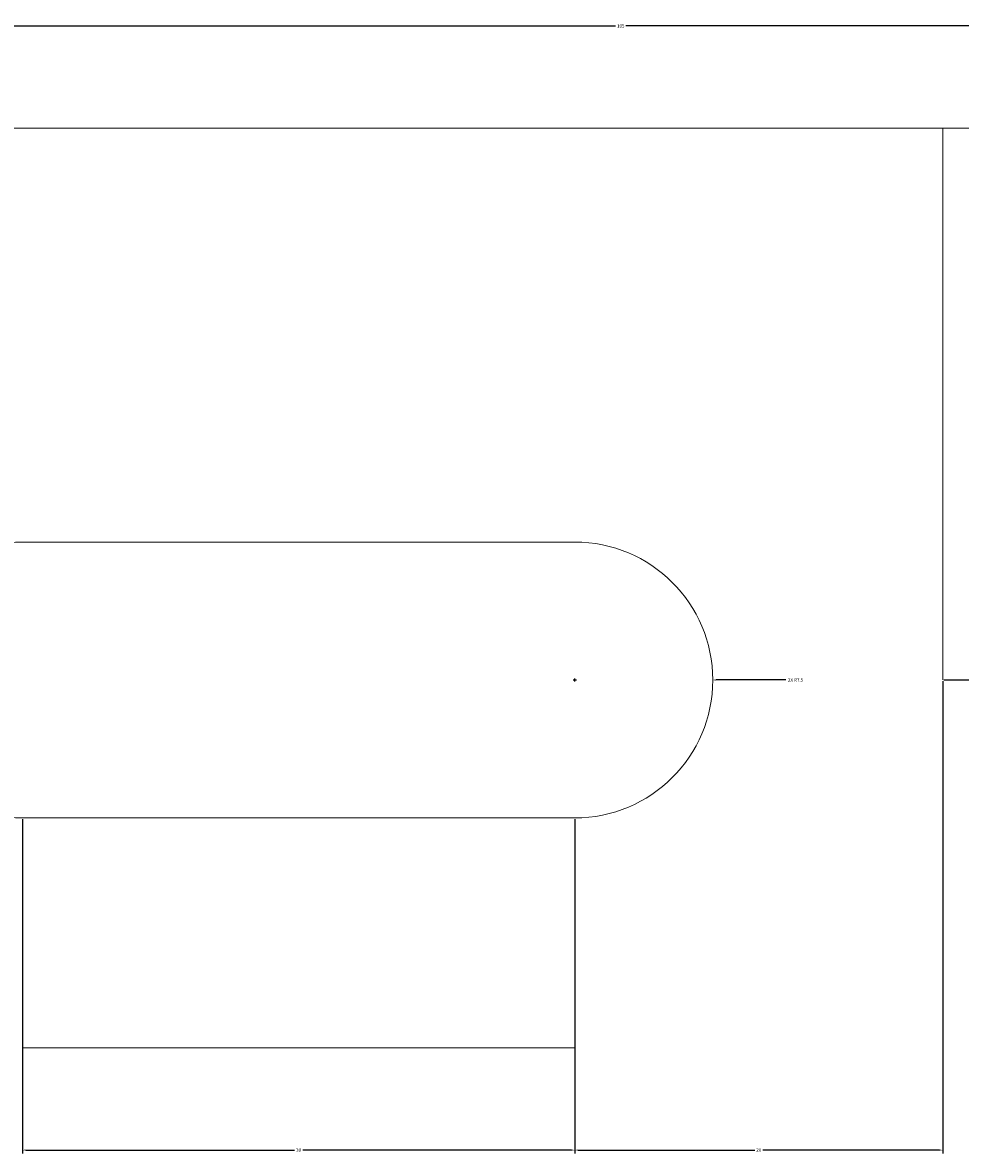
# Model space of a CAD drawing. Units: millimetres. Extents: x 88 to 204, y -56 to 6.
# Tile 2 of 3: x 114 to 165, y -56 to 6. Entities that reach past the tile are written whole.
import ezdxf

# ---------------------------------------------------------------- set-up
doc = ezdxf.new("R2010")
doc.units = ezdxf.units.MM
doc.layers.add('M-CONS', color=8, linetype='Continuous', lineweight=13)
doc.layers.add('M-DIMS', color=2, linetype='Continuous', lineweight=18)
doc.styles.get("Standard").update_dxf_attribs({"font": 'arial.ttf'})
doc.dimstyles.get("Standard").update_dxf_attribs({"dimtxt": 0.18, "dimasz": 0.18, "dimexe": 0.18, "dimexo": 0.0625, "dimgap": 0.09, "dimtad": 0, "dimtih": 1, "dimtoh": 1, "dimdec": 4, "dimzin": 0, "dimdsep": 46, "dimtxsty": 'Standard', "dimcen": 0.09, "dimadec": 0, "dimazin": 0, "dimtfac": 1, "dimtdec": 4, "dimtofl": 0, "dimtmove": 0, "dimatfit": 3, "dimfxl": 1, "dimtolj": 1, "dimtzin": 0, "dimarcsym": 0})

# ---------------------------------------------------------------- blocks, each defined once
blk = doc.blocks.new('*D1')
at = {"layer": 'Defpoints', "color": 0, "transparency": 16777216}
for p in [(198.717, 5.55), (93.717, 0), (198.717, 0)]:
    blk.add_point(p, dxfattribs=at)
at = {"layer": 'M-DIMS', "color": 0, "lineweight": -2, "transparency": 16777216}
for p, q in [((93.717, 0.062), (93.717, 5.73)), ((93.897, 5.55), (145.936, 5.55)), ((198.537, 5.55), (146.498, 5.55)), ((198.717, 0.062), (198.717, 5.73))]:
    blk.add_line(p, q, dxfattribs=at)
at = {"layer": 'M-DIMS', "color": 0, "transparency": 16777216}
for points in [[(93.897, 5.58), (93.897, 5.52), (93.717, 5.55)], [(198.537, 5.58), (198.537, 5.52), (198.717, 5.55)]]:
    blk.add_solid(points, dxfattribs=at)
at = {"layer": 'M-DIMS', "color": 0, "transparency": 16777216, "insert": (146.217, 5.55), "char_height": 0.18, "attachment_point": 5}
blk.add_mtext('\\A1;105', dxfattribs=at)
blk = doc.blocks.new('*D4')
at = {"layer": 'Defpoints', "color": 0, "transparency": 16777216}
for p in [(113.717, -37.5), (143.717, -37.5), (143.717, -55.55)]:
    blk.add_point(p, dxfattribs=at)
at = {"layer": 'M-DIMS', "color": 0, "lineweight": -2, "transparency": 16777216}
for p, q in [((113.717, -37.562), (113.717, -55.73)), ((143.717, -37.562), (143.717, -55.73)), ((113.897, -55.55), (128.498, -55.55)), ((143.537, -55.55), (128.935, -55.55))]:
    blk.add_line(p, q, dxfattribs=at)
at = {"layer": 'M-DIMS', "color": 0, "transparency": 16777216}
for points in [[(113.897, -55.52), (113.897, -55.58), (113.717, -55.55)], [(143.537, -55.52), (143.537, -55.58), (143.717, -55.55)]]:
    blk.add_solid(points, dxfattribs=at)
at = {"layer": 'M-DIMS', "color": 0, "transparency": 16777216, "insert": (128.717, -55.55), "char_height": 0.18, "attachment_point": 5}
blk.add_mtext('\\A1;30', dxfattribs=at)
blk = doc.blocks.new('*D5')
at = {"layer": 'Defpoints', "color": 0, "transparency": 16777216}
for p in [(163.717, -30), (143.717, -50), (163.717, -55.55)]:
    blk.add_point(p, dxfattribs=at)
at = {"layer": 'M-DIMS', "color": 0, "lineweight": -2, "transparency": 16777216}
for p, q in [((163.717, -30.062), (163.717, -55.73)), ((143.717, -50.062), (143.717, -55.73)), ((143.897, -55.55), (153.497, -55.55)), ((163.537, -55.55), (153.937, -55.55))]:
    blk.add_line(p, q, dxfattribs=at)
at = {"layer": 'M-DIMS', "color": 0, "transparency": 16777216}
for points in [[(143.897, -55.52), (143.897, -55.58), (143.717, -55.55)], [(163.537, -55.52), (163.537, -55.58), (163.717, -55.55)]]:
    blk.add_solid(points, dxfattribs=at)
at = {"layer": 'M-DIMS', "color": 0, "transparency": 16777216, "insert": (153.717, -55.55), "char_height": 0.18, "attachment_point": 5}
blk.add_mtext('\\A1;20', dxfattribs=at)
blk = doc.blocks.new('*D6')
at = {"layer": 'Defpoints', "color": 0, "transparency": 16777216}
for p in [(198.717, 0), (163.717, -30), (204.267, -30)]:
    blk.add_point(p, dxfattribs=at)
at = {"layer": 'M-DIMS', "color": 0, "lineweight": -2, "transparency": 16777216}
for p, q in [((198.779, 0), (204.447, 0)), ((204.267, -0.18), (204.267, -14.818)), ((204.267, -29.82), (204.267, -15.182)), ((163.779, -30), (204.447, -30))]:
    blk.add_line(p, q, dxfattribs=at)
at = {"layer": 'M-DIMS', "color": 0, "transparency": 16777216}
for points in [[(204.237, -0.18), (204.297, -0.18), (204.267, 0)], [(204.237, -29.82), (204.297, -29.82), (204.267, -30)]]:
    blk.add_solid(points, dxfattribs=at)
at = {"layer": 'M-DIMS', "color": 0, "transparency": 16777216, "insert": (204.267, -15), "char_height": 0.18, "attachment_point": 5}
blk.add_mtext('\\A1;30', dxfattribs=at)
blk = doc.blocks.new('*D7')
at = {"layer": 'Defpoints', "color": 0, "transparency": 16777216}
for p in [(143.717, -30), (151.217, -30)]:
    blk.add_point(p, dxfattribs=at)
at = {"layer": 'M-DIMS', "color": 0, "lineweight": -2, "transparency": 16777216}
for p, q in [((143.627, -30), (143.807, -30)), ((143.717, -30.09), (143.717, -29.91)), ((155.181, -30), (151.397, -30))]:
    blk.add_line(p, q, dxfattribs=at)
at = {"layer": 'M-DIMS', "color": 0, "transparency": 16777216}
blk.add_solid([(151.397, -29.97), (151.397, -30.03), (151.217, -30)], dxfattribs=at)
at = {"layer": 'M-DIMS', "color": 0, "transparency": 16777216, "insert": (155.717, -30), "char_height": 0.18, "attachment_point": 5}
blk.add_mtext('\\A1;2X R7.5', dxfattribs=at)

msp = doc.modelspace()

# ---------------------------------------------------------------- linework, layer by layer
at = {"layer": 'M-CONS', "extrusion": (0, -1, 0)}
for p, q in [((163.717, 0, 52.588), (93.717, 0, 52.588)), ((93.717, 0, 72.588), (163.717, 0, 72.588)), ((133.717, 0, 152.588), (198.717, 0, 152.588)), ((163.717, 0, 72.588), (163.717, 0, 77.588))]:
    msp.add_line(p, q, dxfattribs=at)
at = {"layer": 'M-CONS'}
for p, q in [((93.717, 0, 62.588), (163.717, 0, 62.588)), ((163.717, 0, 62.588), (163.717, -30, 62.588)), ((143.717, -22.5, 62.588), (113.717, -22.5, 62.588)), ((113.717, -37.5, 62.588), (143.717, -37.5, 62.588)), ((143.717, -50, 62.588), (113.717, -50, 62.588))]:
    msp.add_line(p, q, dxfattribs=at)
for centre, start, end in [((113.717, -30, 62.588), 90, 270), ((143.717, -30, 62.588), 270, 90)]:
    msp.add_arc(centre, 7.5, start, end, dxfattribs=at)

# ---------------------------------------------------------------- dimensions: what is measured, and where the dimension line sits
at = {"layer": 'M-DIMS'}
for base, p1, p2, picture, middle in [((198.717, 5.55), (93.717, 0), (198.717, 0), '*D1', (146.217, 5.55)), ((163.717, -55.55), (143.717, -50), (163.717, -30), '*D5', (153.717, -55.55)), ((143.717, -55.55), (113.717, -37.5), (143.717, -37.5), '*D4', (128.717, -55.55))]:
    dim = msp.add_linear_dim(base=base, p1=p1, p2=p2, dimstyle='Standard', override={"dimdec": 0, "dimlfac": 1, "dimrnd": 0, "dimzin": 0, "dimdsep": 46, "dimlunit": 2}, dxfattribs=at)
    dim.commit()
    dim.dimension.update_dxf_attribs({"geometry": picture, "text_midpoint": middle})
dim = msp.add_linear_dim(base=(204.267, -30), p1=(198.717, 0), p2=(163.717, -30), angle=90, dimstyle='Standard', override={"dimdec": 0, "dimlfac": 1, "dimrnd": 0, "dimzin": 0, "dimdsep": 46, "dimlunit": 2}, dxfattribs=at)
dim.commit()
dim.dimension.update_dxf_attribs({"geometry": '*D6', "text_midpoint": (204.267, -15)})
dim = msp.add_radius_dim(center=(143.717, -30), mpoint=(151.217, -30), text='2X <>', dimstyle='Standard', override={"dimdec": 1, "dimlfac": 1, "dimrnd": 0, "dimzin": 0, "dimdsep": 46, "dimlunit": 2}, dxfattribs=at)
dim.commit()
dim.dimension.update_dxf_attribs({"geometry": '*D7', "text_midpoint": (155.717, -30), "dimtype": 164})

doc.saveas('drawing.dxf')
